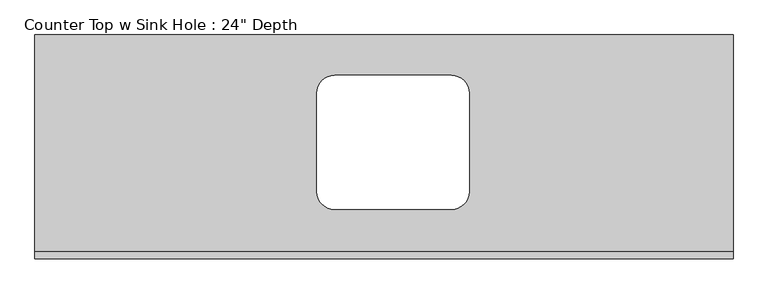
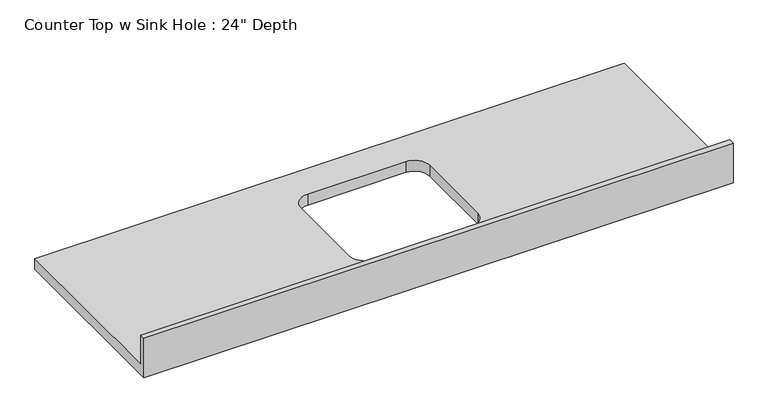
"""IFC4 building model written with IfcOpenShell, lengths in millimetres: furniture geometry."""

from ifc_helpers import new_model, si_unit, frame, origin, place, context, project, spatial, polyline, circle_curve, source, transform, mapped, element, save
from ifc_brep_helpers import plane_surface, revolved_surface, advanced_brep


def furniture_dae9e1b9(model_context):
    return source(origin(), model_context, "Body", "AdvancedBrep", [
        advanced_brep(
        [(-1200.4622951, 635.0, 914.4), (-1200.4622951, 19.05, 914.4), (780.7377049, 19.05, 914.4), (780.7377049, 635.0, 914.4), (-349.5622951, 139.7, 914.4), (-400.3622951, 190.5, 914.4), (-400.3622951, 469.9, 914.4), (-349.5622951, 520.7, 914.4), (-19.3622951, 520.7, 914.4), (31.4377049, 469.9, 914.4), (31.4377049, 190.5, 914.4), (-19.3622951, 139.7, 914.4), (780.7377049, 0.0, 876.3), (-1200.4622951, 0.0, 876.3), (-1200.4622951, 635.0, 876.3), (780.7377049, 635.0, 876.3), (-19.3622951, 139.7, 876.3), (31.4377049, 190.5, 876.3), (31.4377049, 469.9, 876.3), (-19.3622951, 520.7, 876.3), (-349.5622951, 520.7, 876.3), (-400.3622951, 469.9, 876.3), (-400.3622951, 190.5, 876.3), (-349.5622951, 139.7, 876.3), (780.7377049, 0.0, 1016.0), (-1200.4622951, 0.0, 1016.0), (-1200.4622951, 19.05, 1016.0), (780.7377049, 19.05, 1016.0)],
        [
            (0, 1),
            (1, 2),
            (2, 3),
            (3, 0),
            (4, 5, circle_curve(frame((-349.5622951, 190.5, 914.4), z_axis=(0.0, 0.0, -1.0), x_axis=(1.0, 0.0, 0.0)), 50.8)),
            (5, 6),
            (6, 7, circle_curve(frame((-349.5622951, 469.9, 914.4), z_axis=(0.0, 0.0, -1.0), x_axis=(1.0, 0.0, 0.0)), 50.8)),
            (7, 8),
            (8, 9, circle_curve(frame((-19.3622951, 469.9, 914.4), z_axis=(0.0, 0.0, -1.0), x_axis=(1.0, 0.0, 0.0)), 50.8)),
            (9, 10),
            (10, 11, circle_curve(frame((-19.3622951, 190.5, 914.4), z_axis=(0.0, 0.0, -1.0), x_axis=(1.0, 0.0, 0.0)), 50.8)),
            (11, 4),
            (12, 13),
            (13, 14),
            (14, 15),
            (15, 12),
            (16, 17, circle_curve(frame((-19.3622951, 190.5, 876.3), z_axis=(0.0, 0.0, 1.0), x_axis=(1.0, 0.0, 0.0)), 50.8)),
            (17, 18),
            (18, 19, circle_curve(frame((-19.3622951, 469.9, 876.3), z_axis=(0.0, 0.0, 1.0), x_axis=(1.0, 0.0, 0.0)), 50.8)),
            (19, 20),
            (20, 21, circle_curve(frame((-349.5622951, 469.9, 876.3), z_axis=(0.0, 0.0, 1.0), x_axis=(1.0, 0.0, 0.0)), 50.8)),
            (21, 22),
            (22, 23, circle_curve(frame((-349.5622951, 190.5, 876.3), z_axis=(0.0, 0.0, 1.0), x_axis=(1.0, 0.0, 0.0)), 50.8)),
            (23, 16),
            (12, 24),
            (24, 25),
            (25, 13),
            (25, 26),
            (26, 1),
            (0, 14),
            (3, 15),
            (2, 27),
            (27, 24),
            (11, 16),
            (23, 4),
            (22, 5),
            (21, 6),
            (20, 7),
            (19, 8),
            (18, 9),
            (17, 10),
            (27, 26),
        ],
        [
            plane_surface(frame((-1200.4622951, 0.0, 914.4), z_axis=(0.0, 0.0, 1.0), x_axis=(-1.0, 0.0, 0.0))),
            plane_surface(frame((-1200.4622951, 0.0, 876.3), z_axis=(0.0, 0.0, -1.0), x_axis=(1.0, 0.0, 0.0))),
            plane_surface(frame((780.7377049, 0.0, 914.4), z_axis=(0.0, -1.0, 0.0), x_axis=(0.0, 0.0, -1.0))),
            plane_surface(frame((-1200.4622951, 0.0, 914.4), z_axis=(-1.0, 0.0, 0.0), x_axis=(0.0, 0.0, -1.0))),
            plane_surface(frame((-1200.4622951, 635.0, 914.4), z_axis=(0.0, 1.0, 0.0), x_axis=(0.0, 0.0, -1.0))),
            plane_surface(frame((780.7377049, 635.0, 914.4), z_axis=(1.0, 0.0, 0.0), x_axis=(0.0, 0.0, -1.0))),
            plane_surface(frame((-19.3622951, 139.7, 914.4), z_axis=(0.0, 1.0, 0.0), x_axis=(0.0, 0.0, -1.0))),
            revolved_surface(polyline([(-298.76229509999996, 190.5, 914.4), (-298.76229509999996, 190.5, 876.3)]), (-349.5622951, 190.5, 876.3), (0.0, 0.0, 1.0)),
            plane_surface(frame((-400.3622951, 190.5, 914.4), z_axis=(1.0, 0.0, 0.0), x_axis=(0.0, 0.0, -1.0))),
            revolved_surface(polyline([(-298.76229509999996, 469.9, 914.4), (-298.76229509999996, 469.9, 876.3)]), (-349.5622951, 469.9, 876.3), (0.0, 0.0, 1.0)),
            plane_surface(frame((-349.5622951, 520.7, 914.4), z_axis=(0.0, -1.0, 0.0), x_axis=(0.0, 0.0, -1.0))),
            revolved_surface(polyline([(31.437704899999996, 469.9, 914.4), (31.437704899999996, 469.9, 876.3)]), (-19.3622951, 469.9, 876.3), (0.0, 0.0, 1.0)),
            plane_surface(frame((31.4377049, 469.9, 914.4), z_axis=(-1.0, 0.0, 0.0), x_axis=(0.0, 0.0, -1.0))),
            revolved_surface(polyline([(31.437704899999996, 190.5, 914.4), (31.437704899999996, 190.5, 876.3)]), (-19.3622951, 190.5, 876.3), (0.0, 0.0, 1.0)),
            plane_surface(frame((-1200.4622951, 0.0, 1016.0), z_axis=(0.0, 0.0, 1.0), x_axis=(0.0, 1.0, 0.0))),
            plane_surface(frame((-1200.4622951, 19.05, 1016.0), z_axis=(0.0, 1.0, 0.0), x_axis=(0.0, 0.0, -1.0))),
        ],
        [
            (0, [[1, 2, 3, 4], [5, 6, 7, 8, 9, 10, 11, 12]]),
            (1, [[13, 14, 15, 16], [17, 18, 19, 20, 21, 22, 23, 24]]),
            (2, [[25, 26, 27, -13]]),
            (3, [[-27, 28, 29, -1, 30, -14]]),
            (4, [[31, -15, -30, -4]]),
            (5, [[-31, -3, 32, 33, -25, -16]]),
            (6, [[-12, 34, -24, 35]]),
            (7, [[-23, 36, -5, -35]]),
            (8, [[-22, 37, -6, -36]]),
            (9, [[-21, 38, -7, -37]]),
            (10, [[-20, 39, -8, -38]]),
            (11, [[-19, 40, -9, -39]]),
            (12, [[-18, 41, -10, -40]]),
            (13, [[-11, -41, -17, -34]]),
            (14, [[-26, -33, 42, -28]]),
            (15, [[-32, -2, -29, -42]]),
        ],
    ),
    ])


if __name__ == "__main__":
    model = new_model("IFC4")
    model_context = context("Model", 3, world=origin())
    ifc_project = project(units=[si_unit("LENGTHUNIT", "METRE", prefix="MILLI")], contexts=[model_context])
    site = spatial("IfcSite", under=ifc_project)
    building = spatial("IfcBuilding", under=site)
    placement = place(None, origin())
    furniture_shape = furniture_dae9e1b9(model_context)
    element("IfcFurniture", 1, ObjectType="Counter Top w Sink Hole : 24\" Depth", at=placement, inside=building, context=model_context, shape_type="MappedRepresentation", body=[
        mapped(furniture_shape, transform((0.0, 0.0, 0.0), x_axis=(1.0, 0.0, 0.0), y_axis=(0.0, 1.0, 0.0), z_axis=(0.0, 0.0, 1.0))),
    ])
    save(model, "model.ifc")

# Revit data of these elements
# Type "Counter Top w Sink Hole : 24\" Depth"
#   Assembly Code = "C1030400"
#   Counter Thickness = 0' - 1 1/2"
#   Depth = 2' - 1"
#   Height = 3' - 0"
#   Length [instance default] = 8' - 0"
#   Sink Location [instance default] = 2' - 0"
#   Sink Location To Wall [instance default] = 0' - 6"
#   Sink Opening Depth [instance default] = 1' - 3"
#   Sink Opening Width [instance default] = 2' - 3"
#   Counter Top Material = none
#   Default Elevation = 0
# Element 1 (IfcFurniture, "Counter Top w Sink Hole : 24\" Depth")
#   Length = 6' - 6"
#   Sink Location = 3' - 4"
#   Sink Opening Depth = 1' - 2"
#   Sink Opening Width = 1' - 4"
#   Materials on its faces: "Counter Top"
# Materials
#   "Counter Top": class "Wood", colour RGB 226 177 128, transparency 0
